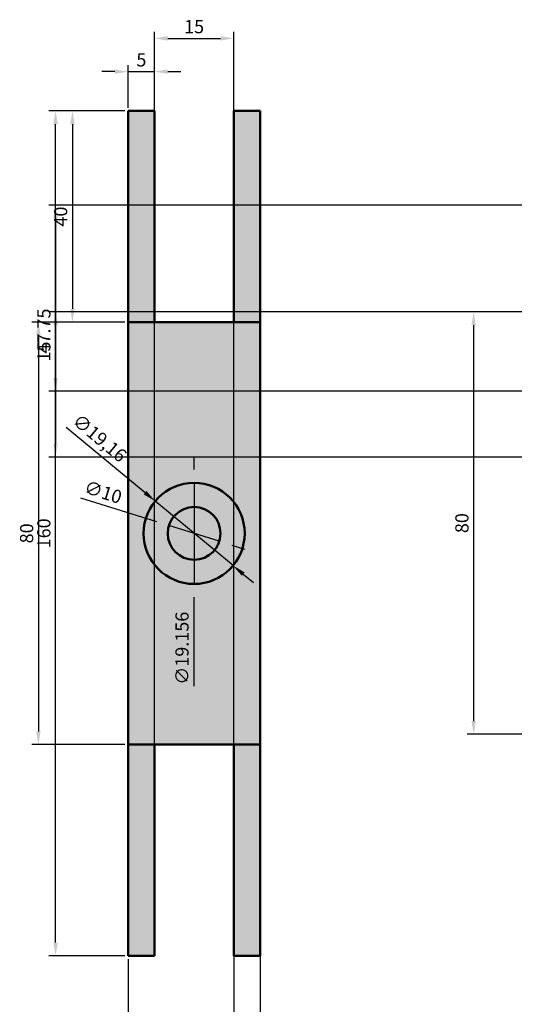
# Model space of a CAD drawing. Units: millimetres. Extents: x 2180 to 2428, y 1025 to 1371.
# Tile 2 of 3: x 2180 to 2274, y 1185 to 1371. Entities that reach past the tile are written whole.
import ezdxf

# ---------------------------------------------------------------- set-up
doc = ezdxf.new("R2010")
doc.units = ezdxf.units.MM
for name, color, linetype, lineweight in [('M-DIMS', 2, 'Continuous', 25), ('M-HATC', 252, 'Continuous', 18), ('M-OUTL', 7, 'Continuous', 50)]:
    doc.layers.add(name, color=color, linetype=linetype, lineweight=lineweight)
doc.styles.get("Standard").update_dxf_attribs({"font": 'arial.ttf'})
doc.dimstyles.new('ISO-25', dxfattribs={"dimtxt": 2.5, "dimasz": 2.5, "dimexe": 1.25, "dimexo": 0.625, "dimtad": 1, "dimtxsty": 'Standard', "dimcen": 2.5, "dimadec": 0, "dimazin": 0, "dimtfac": 1, "dimtmove": 0, "dimatfit": 3, "dimfxl": 1, "dimarcsym": 0})

# ---------------------------------------------------------------- blocks, each defined once
blk = doc.blocks.new('*D1')
at = {"layer": 'Defpoints', "color": 0, "transparency": 16777216}
for p in [(2200.82, 1314.18), (2183.81, 1234.18), (2200.82, 1234.18)]:
    blk.add_point(p, dxfattribs=at)
at = {"layer": 'M-DIMS', "color": 0, "lineweight": -2, "transparency": 16777216}
for p, q in [((2200.19, 1314.18), (2182.56, 1314.18)), ((2183.81, 1311.68), (2183.81, 1236.68)), ((2200.19, 1234.18), (2182.56, 1234.18))]:
    blk.add_line(p, q, dxfattribs=at)
at = {"layer": 'M-DIMS', "color": 0, "transparency": 16777216}
for points in [[(2183.39, 1311.68), (2184.23, 1311.68), (2183.81, 1314.18)], [(2183.39, 1236.68), (2184.23, 1236.68), (2183.81, 1234.18)]]:
    blk.add_solid(points, dxfattribs=at)
at = {"layer": 'M-DIMS', "color": 0, "transparency": 16777216, "insert": (2181.91, 1274.18), "char_height": 2.5, "attachment_point": 5, "rotation": 90}
blk.add_mtext('80', dxfattribs=at)
blk = doc.blocks.new('*D2')
at = {"layer": 'Defpoints', "color": 0, "transparency": 16777216}
for p in [(2205.82, 1361.63), (2200.82, 1354.18), (2205.82, 1354.18)]:
    blk.add_point(p, dxfattribs=at)
at = {"layer": 'M-DIMS', "color": 0, "lineweight": -2, "transparency": 16777216}
for p, q in [((2198.32, 1361.63), (2195.82, 1361.63)), ((2200.82, 1354.8), (2200.82, 1362.88)), ((2200.82, 1361.63), (2205.82, 1361.63)), ((2205.82, 1354.8), (2205.82, 1362.88)), ((2208.32, 1361.63), (2210.82, 1361.63))]:
    blk.add_line(p, q, dxfattribs=at)
at = {"layer": 'M-DIMS', "color": 0, "transparency": 16777216}
for points in [[(2198.32, 1362.05), (2198.32, 1361.21), (2200.82, 1361.63)], [(2208.32, 1362.05), (2208.32, 1361.21), (2205.82, 1361.63)]]:
    blk.add_solid(points, dxfattribs=at)
at = {"layer": 'M-DIMS', "color": 0, "transparency": 16777216, "insert": (2203.32, 1363.53), "char_height": 2.5, "attachment_point": 5}
blk.add_mtext('5', dxfattribs=at)
blk = doc.blocks.new('*D3')
at = {"layer": 'Defpoints', "color": 0, "transparency": 16777216}
for p in [(2200.82, 1354.18), (2190.26, 1314.18), (2200.82, 1314.18)]:
    blk.add_point(p, dxfattribs=at)
at = {"layer": 'M-DIMS', "color": 0, "lineweight": -2, "transparency": 16777216}
for p, q in [((2200.19, 1354.18), (2189.01, 1354.18)), ((2190.26, 1351.68), (2190.26, 1316.68)), ((2200.19, 1314.18), (2189.01, 1314.18))]:
    blk.add_line(p, q, dxfattribs=at)
at = {"layer": 'M-DIMS', "color": 0, "transparency": 16777216}
for points in [[(2189.85, 1351.68), (2190.68, 1351.68), (2190.26, 1354.18)], [(2189.85, 1316.68), (2190.68, 1316.68), (2190.26, 1314.18)]]:
    blk.add_solid(points, dxfattribs=at)
at = {"layer": 'M-DIMS', "color": 0, "transparency": 16777216, "insert": (2188.36, 1334.18), "char_height": 2.5, "attachment_point": 5, "rotation": 90}
blk.add_mtext('40', dxfattribs=at)
blk = doc.blocks.new('*D4')
at = {"layer": 'Defpoints', "color": 0, "transparency": 16777216}
for p in [(2208.55, 1275.68), (2218.09, 1272.68)]:
    blk.add_point(p, dxfattribs=at)
at = {"layer": 'M-DIMS', "color": 0, "lineweight": -2, "transparency": 16777216}
for p, q in [((2191.79, 1280.94), (2206.16, 1276.43)), ((2218.09, 1272.68), (2208.55, 1275.68)), ((2220.47, 1271.93), (2222.86, 1271.18))]:
    blk.add_line(p, q, dxfattribs=at)
at = {"layer": 'M-DIMS', "color": 0, "transparency": 16777216}
for points in [[(2206.29, 1276.82), (2206.04, 1276.03), (2208.55, 1275.68)], [(2220.6, 1272.33), (2220.35, 1271.53), (2218.09, 1272.68)]]:
    blk.add_solid(points, dxfattribs=at)
at = {"layer": 'M-DIMS', "color": 0, "transparency": 16777216, "insert": (2195.98, 1281.69), "char_height": 2.5, "attachment_point": 5, "rotation": 342.5609}
blk.add_mtext('∅10', dxfattribs=at)
blk = doc.blocks.new('*D5')
at = {"layer": 'Defpoints', "color": 0, "transparency": 16777216}
for p in [(2205.94, 1280.29), (2220.69, 1268.07)]:
    blk.add_point(p, dxfattribs=at)
at = {"layer": 'M-DIMS', "color": 0, "lineweight": -2, "transparency": 16777216}
for p, q in [((2189.07, 1294.28), (2204.02, 1281.89)), ((2220.69, 1268.07), (2205.94, 1280.29)), ((2222.62, 1266.47), (2224.54, 1264.88))]:
    blk.add_line(p, q, dxfattribs=at)
at = {"layer": 'M-DIMS', "color": 0, "transparency": 16777216}
for points in [[(2204.29, 1282.21), (2203.75, 1281.57), (2205.94, 1280.29)], [(2222.88, 1266.79), (2222.35, 1266.15), (2220.69, 1268.07)]]:
    blk.add_solid(points, dxfattribs=at)
at = {"layer": 'M-DIMS', "color": 0, "transparency": 16777216, "insert": (2195.23, 1291.99), "char_height": 2.5, "attachment_point": 5, "rotation": 320.3456}
blk.add_mtext('∅19,16', dxfattribs=at)
blk = doc.blocks.new('*D6')
at = {"layer": 'Defpoints', "color": 0, "transparency": 16777216}
for p in [(2290.36, 1316.12), (2266.28, 1236.12), (2290.36, 1236.12)]:
    blk.add_point(p, dxfattribs=at)
at = {"layer": 'M-DIMS', "color": 0, "lineweight": -2, "transparency": 16777216}
for p, q in [((2289.74, 1316.12), (2265.03, 1316.12)), ((2266.28, 1313.62), (2266.28, 1238.62)), ((2289.74, 1236.12), (2265.03, 1236.12))]:
    blk.add_line(p, q, dxfattribs=at)
at = {"layer": 'M-DIMS', "color": 0, "transparency": 16777216}
for points in [[(2265.87, 1313.62), (2266.7, 1313.62), (2266.28, 1316.12)], [(2265.87, 1238.62), (2266.7, 1238.62), (2266.28, 1236.12)]]:
    blk.add_solid(points, dxfattribs=at)
at = {"layer": 'M-DIMS', "color": 0, "transparency": 16777216, "insert": (2264.38, 1276.12), "char_height": 2.5, "attachment_point": 5, "rotation": 90}
blk.add_mtext('80', dxfattribs=at)
blk = doc.blocks.new('*D30')
at = {"layer": 'Defpoints', "color": 0, "transparency": 16777216}
for p in [(2200.82, 1194.18), (2225.82, 1194.18), (2225.82, 1089.54)]:
    blk.add_point(p, dxfattribs=at)
at = {"layer": 'M-DIMS', "color": 0, "lineweight": -2, "transparency": 16777216}
for p, q in [((2200.82, 1193.55), (2200.82, 1088.29)), ((2225.82, 1193.55), (2225.82, 1088.29)), ((2203.32, 1089.54), (2223.32, 1089.54))]:
    blk.add_line(p, q, dxfattribs=at)
at = {"layer": 'M-DIMS', "color": 0, "transparency": 16777216}
for points in [[(2203.32, 1089.96), (2203.32, 1089.12), (2200.82, 1089.54)], [(2223.32, 1089.96), (2223.32, 1089.12), (2225.82, 1089.54)]]:
    blk.add_solid(points, dxfattribs=at)
at = {"layer": 'M-DIMS', "color": 0, "transparency": 16777216, "insert": (2213.32, 1091.44), "char_height": 2.5, "attachment_point": 5}
blk.add_mtext('25', dxfattribs=at)
blk = doc.blocks.new('*D31')
at = {"layer": 'Defpoints', "color": 0, "transparency": 16777216}
for p in [(2187.07, 1354.18), (2200.82, 1354.18), (2200.82, 1194.18)]:
    blk.add_point(p, dxfattribs=at)
at = {"layer": 'M-DIMS', "color": 0, "lineweight": -2, "transparency": 16777216}
for p, q in [((2200.19, 1354.18), (2185.82, 1354.18)), ((2187.07, 1196.68), (2187.07, 1351.68)), ((2200.19, 1194.18), (2185.82, 1194.18))]:
    blk.add_line(p, q, dxfattribs=at)
at = {"layer": 'M-DIMS', "color": 0, "transparency": 16777216}
for points in [[(2186.65, 1351.68), (2187.49, 1351.68), (2187.07, 1354.18)], [(2186.65, 1196.68), (2187.49, 1196.68), (2187.07, 1194.18)]]:
    blk.add_solid(points, dxfattribs=at)
at = {"layer": 'M-DIMS', "color": 0, "transparency": 16777216, "insert": (2185.17, 1274.18), "char_height": 2.5, "attachment_point": 5, "rotation": 90}
blk.add_mtext('160', dxfattribs=at)
blk = doc.blocks.new('*D32')
at = {"layer": 'Defpoints', "color": 0, "transparency": 16777216}
for p in [(2220.82, 1367.93), (2205.82, 1354.18), (2220.82, 1354.18)]:
    blk.add_point(p, dxfattribs=at)
at = {"layer": 'M-DIMS', "color": 0, "lineweight": -2, "transparency": 16777216}
for p, q in [((2205.82, 1354.8), (2205.82, 1369.18)), ((2220.82, 1354.8), (2220.82, 1369.18)), ((2208.32, 1367.93), (2218.32, 1367.93))]:
    blk.add_line(p, q, dxfattribs=at)
at = {"layer": 'M-DIMS', "color": 0, "transparency": 16777216}
for points in [[(2208.32, 1368.35), (2208.32, 1367.51), (2205.82, 1367.93)], [(2218.32, 1368.35), (2218.32, 1367.51), (2220.82, 1367.93)]]:
    blk.add_solid(points, dxfattribs=at)
at = {"layer": 'M-DIMS', "color": 0, "transparency": 16777216, "insert": (2213.32, 1369.83), "char_height": 2.5, "attachment_point": 5}
blk.add_mtext('15', dxfattribs=at)
blk = doc.blocks.new('*D33')
at = {"layer": 'Defpoints', "color": 0, "transparency": 16777216}
for p in [(2220.82, 1367.93), (2205.82, 1194.18), (2220.82, 1194.18)]:
    blk.add_point(p, dxfattribs=at)
at = {"layer": 'M-DIMS', "color": 0, "lineweight": -2, "transparency": 16777216}
for p, q in [((2205.82, 1194.8), (2205.82, 1369.18)), ((2220.82, 1194.8), (2220.82, 1369.18)), ((2208.32, 1367.93), (2218.32, 1367.93))]:
    blk.add_line(p, q, dxfattribs=at)
at = {"layer": 'M-DIMS', "color": 0, "transparency": 16777216}
for points in [[(2208.32, 1368.35), (2208.32, 1367.51), (2205.82, 1367.93)], [(2218.32, 1368.35), (2218.32, 1367.51), (2220.82, 1367.93)]]:
    blk.add_solid(points, dxfattribs=at)
at = {"layer": 'M-DIMS', "color": 0, "transparency": 16777216, "insert": (2213.32, 1369.83), "char_height": 2.5, "attachment_point": 5}
blk.add_mtext('15', dxfattribs=at)
blk = doc.blocks.new('*D34')
at = {"layer": 'Defpoints', "color": 0, "transparency": 16777216}
for p in [(2220.82, 1234.18), (2225.82, 1234.18), (2225.82, 1089.54)]:
    blk.add_point(p, dxfattribs=at)
at = {"layer": 'M-DIMS', "color": 0, "lineweight": -2, "transparency": 16777216}
for p, q in [((2220.82, 1233.55), (2220.82, 1088.29)), ((2225.82, 1233.55), (2225.82, 1088.29)), ((2218.32, 1089.54), (2215.82, 1089.54)), ((2220.82, 1089.54), (2225.82, 1089.54)), ((2228.32, 1089.54), (2230.82, 1089.54))]:
    blk.add_line(p, q, dxfattribs=at)
at = {"layer": 'M-DIMS', "color": 0, "transparency": 16777216}
for points in [[(2218.32, 1089.96), (2218.32, 1089.12), (2220.82, 1089.54)], [(2228.32, 1089.96), (2228.32, 1089.12), (2225.82, 1089.54)]]:
    blk.add_solid(points, dxfattribs=at)
at = {"layer": 'M-DIMS', "color": 0, "transparency": 16777216, "insert": (2223.32, 1091.44), "char_height": 2.5, "attachment_point": 5}
blk.add_mtext('5', dxfattribs=at)
blk = doc.blocks.new('*D36')
at = {"layer": 'Defpoints', "color": 0, "transparency": 16777216}
for p in [(2386.95, 1336.37), (2187.07, 1288.62), (2407.33, 1288.62)]:
    blk.add_point(p, dxfattribs=at)
at = {"layer": 'M-DIMS', "color": 0, "lineweight": -2, "transparency": 16777216}
for p, q in [((2386.33, 1336.37), (2185.82, 1336.37)), ((2187.07, 1333.87), (2187.07, 1291.12)), ((2406.71, 1288.62), (2185.82, 1288.62))]:
    blk.add_line(p, q, dxfattribs=at)
at = {"layer": 'M-DIMS', "color": 0, "transparency": 16777216}
for points in [[(2186.65, 1333.87), (2187.49, 1333.87), (2187.07, 1336.37)], [(2186.65, 1291.12), (2187.49, 1291.12), (2187.07, 1288.62)]]:
    blk.add_solid(points, dxfattribs=at)
at = {"layer": 'M-DIMS', "color": 0, "transparency": 16777216, "insert": (2185.17, 1312.5), "char_height": 2.5, "attachment_point": 5, "rotation": 90}
blk.add_mtext('47.75', dxfattribs=at)
blk = doc.blocks.new('*D40')
at = {"layer": 'Defpoints', "color": 0, "transparency": 16777216}
for p in [(2290.36, 1316.12), (2187.07, 1301.12), (2294.36, 1301.12)]:
    blk.add_point(p, dxfattribs=at)
at = {"layer": 'M-DIMS', "color": 0, "lineweight": -2, "transparency": 16777216}
for p, q in [((2289.74, 1316.12), (2185.82, 1316.12)), ((2187.07, 1313.62), (2187.07, 1303.62)), ((2293.74, 1301.12), (2185.82, 1301.12))]:
    blk.add_line(p, q, dxfattribs=at)
at = {"layer": 'M-DIMS', "color": 0, "transparency": 16777216}
for points in [[(2186.65, 1313.62), (2187.49, 1313.62), (2187.07, 1316.12)], [(2186.65, 1303.62), (2187.49, 1303.62), (2187.07, 1301.12)]]:
    blk.add_solid(points, dxfattribs=at)
at = {"layer": 'M-DIMS', "color": 0, "transparency": 16777216, "insert": (2185.17, 1308.62), "char_height": 2.5, "attachment_point": 5, "rotation": 90}
blk.add_mtext('15', dxfattribs=at)
blk = doc.blocks.new('*D47')
at = {"layer": 'Defpoints', "color": 0, "transparency": 16777216}
for p in [(2213.32, 1283.76), (2213.32, 1264.6)]:
    blk.add_point(p, dxfattribs=at)
at = {"layer": 'M-DIMS', "color": 0, "lineweight": -2, "transparency": 16777216}
for p, q in [((2213.32, 1286.26), (2213.32, 1288.76)), ((2213.32, 1283.76), (2213.32, 1264.6)), ((2213.32, 1245.25), (2213.32, 1262.1))]:
    blk.add_line(p, q, dxfattribs=at)
at = {"layer": 'M-DIMS', "color": 0, "transparency": 16777216}
for points in [[(2212.9, 1286.26), (2213.74, 1286.26), (2213.32, 1283.76)], [(2212.9, 1262.1), (2213.74, 1262.1), (2213.32, 1264.6)]]:
    blk.add_solid(points, dxfattribs=at)
at = {"layer": 'M-DIMS', "color": 0, "transparency": 16777216, "insert": (2211.35, 1252.43), "char_height": 2.5, "attachment_point": 5, "rotation": 89.999}
blk.add_mtext('∅19.156', dxfattribs=at)

msp = doc.modelspace()

# ---------------------------------------------------------------- hatches: boundary and pattern name
at = {"layer": 'M-HATC'}
h = msp.add_hatch(color=256, dxfattribs=at)
h.set_gradient(color1=(100, 33, 101), color2=(100, 33, 101), tint=1)
h.paths.add_polyline_path([(2225.8192, 1354.1795), (2220.8192, 1354.1795), (2220.8192, 1314.1795), (2225.8192, 1314.1795)])
h.paths.add_polyline_path([(2205.8192, 1354.1795), (2200.8192, 1354.1795), (2200.8192, 1314.1795), (2205.8192, 1314.1795)])
h.paths.add_polyline_path([(2225.8192, 1314.1795), (2220.8192, 1314.1795), (2200.8192, 1314.1795), (2200.8192, 1234.1795), (2205.8192, 1234.1795), (2225.8192, 1234.1795)])
h.paths.add_polyline_path([(2222.8972, 1274.1795, -1), (2203.7411, 1274.1795, -1)], flags=0)
h.paths.add_polyline_path([(2218.3192, 1274.1795, -1), (2208.3192, 1274.1795, -1)], flags=0)
h.paths.add_polyline_path([(2205.8192, 1234.1795), (2200.8192, 1234.1795), (2200.8192, 1194.1795), (2205.8192, 1194.1795)])
h.paths.add_polyline_path([(2225.8192, 1234.1795), (2220.8192, 1234.1795), (2220.8192, 1194.1795), (2225.8192, 1194.1795)])
h.paths.add_polyline_path([(2203.7411, 1274.1795, 1), (2222.8972, 1274.1795, 1)], flags=16)
h.paths.add_polyline_path([(2208.3192, 1274.1795, 1), (2218.3192, 1274.1795, 1)], flags=0)

# ---------------------------------------------------------------- linework, layer by layer
at = {"layer": 'M-OUTL'}
for p, q in [((2205.8192, 1354.1795), (2200.8192, 1354.1795)), ((2200.8192, 1354.1795), (2200.8192, 1314.1795)), ((2205.8192, 1314.1795), (2205.8192, 1354.1795)), ((2220.8192, 1314.1795), (2220.8192, 1354.1795)), ((2220.8192, 1354.1795), (2225.8192, 1354.1795)), ((2225.8192, 1354.1795), (2225.8192, 1314.1795)), ((2200.8192, 1314.1795), (2225.8192, 1314.1795)), ((2200.8192, 1234.1795), (2200.8192, 1314.1795)), ((2200.8192, 1314.1795), (2205.8192, 1314.1795)), ((2225.8192, 1314.1795), (2220.8192, 1314.1795)), ((2225.8192, 1314.1795), (2225.8192, 1234.1795)), ((2225.8192, 1234.1795), (2200.8192, 1234.1795)), ((2200.8192, 1234.1795), (2205.8192, 1234.1795)), ((2200.8192, 1194.1795), (2200.8192, 1234.1795)), ((2205.8192, 1234.1795), (2205.8192, 1194.1795)), ((2225.8192, 1234.1795), (2220.8192, 1234.1795)), ((2220.8192, 1234.1795), (2220.8192, 1194.1795)), ((2225.8192, 1194.1795), (2225.8192, 1234.1795)), ((2205.8192, 1194.1795), (2200.8192, 1194.1795)), ((2220.8192, 1194.1795), (2225.8192, 1194.1795))]:
    msp.add_line(p, q, dxfattribs=at)
for radius in [9.5781, 5]:
    msp.add_circle((2213.3192, 1274.1795), radius, dxfattribs=at)

# ---------------------------------------------------------------- dimensions: what is measured, and where the dimension line sits
at = {"layer": 'M-DIMS'}
for base, p1, p2, override, picture, middle in [((2220.8192, 1367.9295), (2205.8192, 1354.1795), (2220.8192, 1354.1795), {"dimdec": 0, "dimlfac": 1, "dimrnd": 0, "dimzin": 0, "dimdsep": 46, "dimlunit": 2}, '*D32', (2213.3192, 1369.831)), ((2220.8192, 1367.9295), (2205.8192, 1194.1795), (2220.8192, 1194.1795), {"dimdec": 0, "dimlfac": 1, "dimrnd": 0, "dimzin": 0, "dimdsep": 46, "dimlunit": 2}, '*D33', (2213.3192, 1369.831)), ((2205.8192, 1361.63), (2200.8192, 1354.1795), (2205.8192, 1354.1795), {"dimclrd": 0, "dimclre": 0, "dimclrt": 0}, '*D2', (2203.3192, 1363.5263)), ((2225.8192, 1089.5404), (2220.8192, 1234.1795), (2225.8192, 1234.1795), {"dimdec": 0, "dimlfac": 1, "dimrnd": 0, "dimzin": 0, "dimdsep": 46, "dimlunit": 2}, '*D34', (2223.3192, 1091.4367)), ((2225.8192, 1089.5404), (2200.8192, 1194.1795), (2225.8192, 1194.1795), {"dimdec": 0, "dimlfac": 1, "dimrnd": 0, "dimzin": 0, "dimdsep": 46, "dimlunit": 2}, '*D30', (2213.3192, 1091.4418))]:
    dim = msp.add_linear_dim(base=base, p1=p1, p2=p2, dimstyle='ISO-25', override=override, dxfattribs=at)
    dim.commit()
    dim.dimension.update_dxf_attribs({"geometry": picture, "text_midpoint": middle})
for base, p1, p2, override, picture, middle in [((2187.0692, 1354.1795), (2200.8192, 1194.1795), (2200.8192, 1354.1795), {"dimdec": 0, "dimlfac": 1, "dimrnd": 0, "dimzin": 0, "dimdsep": 46, "dimlunit": 2}, '*D31', (2185.1677, 1274.1795)), ((2190.2648, 1314.1795), (2200.8192, 1354.1795), (2200.8192, 1314.1795), {"dimclrd": 0, "dimclre": 0, "dimclrt": 0}, '*D3', (2188.3634, 1334.1795)), ((2187.0692, 1288.625), (2386.9536, 1336.3721), (2407.3324, 1288.625), {"dimdec": 2, "dimlfac": 1, "dimrnd": 0, "dimzin": 0, "dimdsep": 46, "dimlunit": 2}, '*D36', (2185.1728, 1312.4986)), ((2187.0692, 1301.125), (2290.3614, 1316.125), (2294.3614, 1301.125), {"dimdec": 0, "dimlfac": 1, "dimrnd": 0, "dimzin": 0, "dimdsep": 46, "dimlunit": 2}, '*D40', (2185.1677, 1308.625)), ((2266.283, 1236.125), (2290.3614, 1316.125), (2290.3614, 1236.125), {"dimclrd": 0, "dimclre": 0, "dimclrt": 0}, '*D6', (2264.3816, 1276.125)), ((2183.8093, 1234.1795), (2200.8192, 1314.1795), (2200.8192, 1234.1795), {"dimclrd": 0, "dimclre": 0, "dimclrt": 0}, '*D1', (2181.9079, 1274.1795))]:
    dim = msp.add_linear_dim(base=base, p1=p1, p2=p2, angle=90, dimstyle='ISO-25', override=override, dxfattribs=at)
    dim.commit()
    dim.dimension.update_dxf_attribs({"geometry": picture, "text_midpoint": middle})
for p1, p2, override, picture, middle in [((2220.6934, 1268.0672), (2205.9449, 1280.2918), {"dimclrd": 0, "dimclre": 0, "dimclrt": 0}, '*D5', (2193.8485, 1290.3182)), ((2213.3193, 1283.7576), (2213.319, 1264.6014), {"dimdec": 3, "dimlfac": 1, "dimrnd": 0, "dimzin": 0, "dimdsep": 46, "dimlunit": 2}, '*D47', (2213.3188, 1252.428)), ((2218.0893, 1272.6811), (2208.549, 1275.678), {"dimclrd": 0, "dimclre": 0, "dimclrt": 0}, '*D4', (2195.3908, 1279.8114))]:
    dim = msp.add_diameter_dim_2p(p1=p1, p2=p2, dimstyle='ISO-25', override=override, dxfattribs=at)
    dim.commit()
    dim.dimension.update_dxf_attribs({"geometry": picture, "text_midpoint": middle, "dimtype": 163})

doc.saveas('drawing.dxf')
